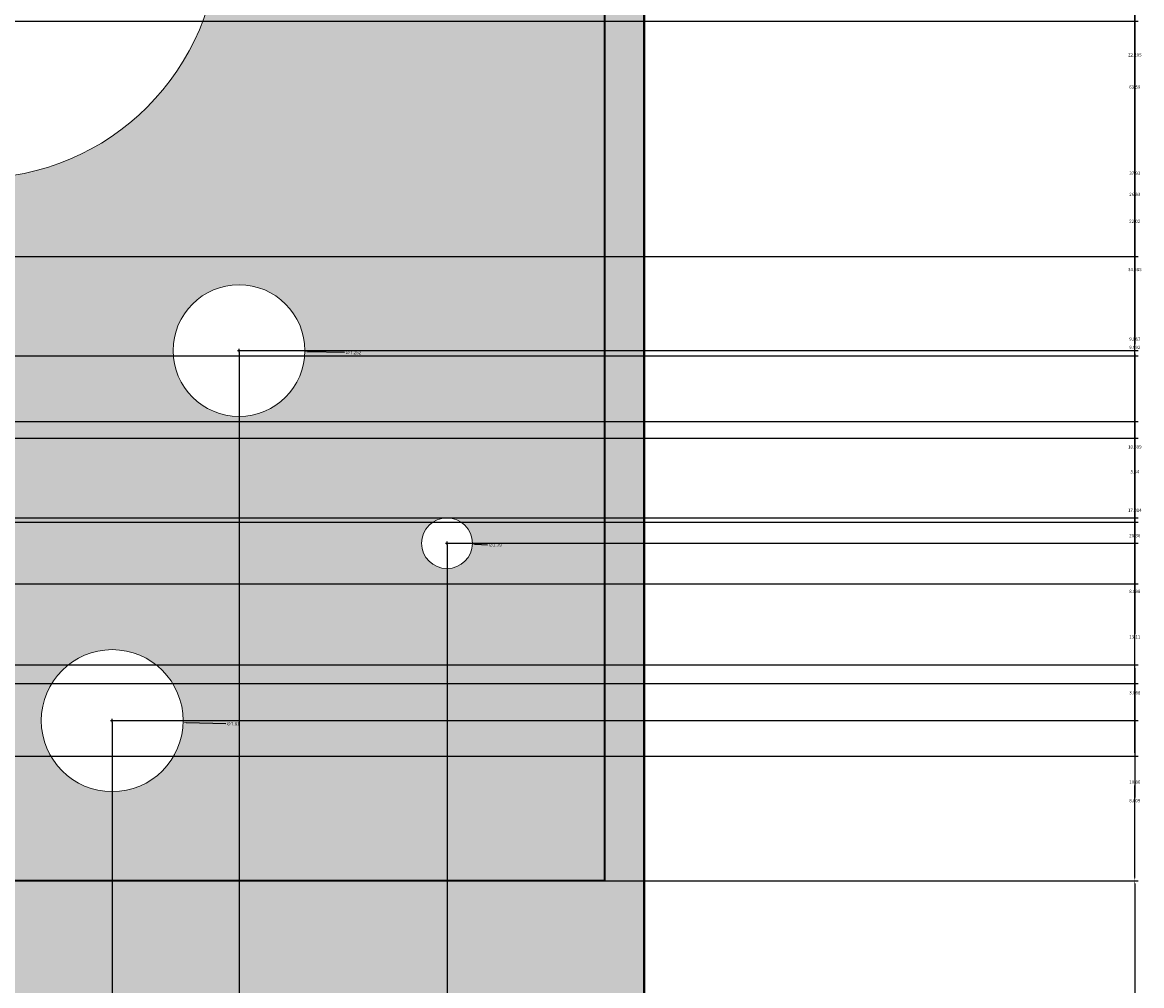
# Model space of a CAD drawing. Units: inches. Extents: x 73 to 607, y 92 to 651.
# Tile 10 of 18: x 546 to 607, y 169 to 222. Entities that reach past the tile are written whole.
import ezdxf

# ---------------------------------------------------------------- set-up
doc = ezdxf.new("R2010")
doc.units = ezdxf.units.IN
doc.header["$MEASUREMENT"] = 0
for name, color, linetype, lineweight in [('A-ANNO-DIMS', 2, 'Continuous', 18), ('A-ELEV', 7, 'Continuous', 35), ('A-ELEV-PANL', 7, 'Continuous', 18), ('A-ELEV-PATT-BKGD', 252, 'Continuous', 13), ('A-ELEV-PATT-SHAD', 8, 'Continuous', 13), ('A-ELEV-PATT-WOOD', 32, 'Continuous', 13)]:
    doc.layers.add(name, color=color, linetype=linetype, lineweight=lineweight)
doc.styles.get("Standard").update_dxf_attribs({"font": 'arial.ttf'})
doc.dimstyles.get("Standard").update_dxf_attribs({"dimtxt": 0.18, "dimasz": 0.18, "dimexe": 0.18, "dimexo": 0.0625, "dimgap": 0.09, "dimtad": 0, "dimtih": 1, "dimtoh": 1, "dimdec": 4, "dimzin": 0, "dimdsep": 46, "dimtxsty": 'Standard', "dimcen": 0.09, "dimadec": 0, "dimazin": 0, "dimtfac": 1, "dimtdec": 4, "dimtofl": 0, "dimtmove": 0, "dimatfit": 3, "dimfxl": 1, "dimtolj": 1, "dimtzin": 0, "dimarcsym": 0})

# ---------------------------------------------------------------- blocks, each defined once
blk = doc.blocks.new('*D15')
at = {"layer": 'A-ANNO-DIMS', "color": 0, "lineweight": -2, "transparency": 16777216}
for p, q in [((454.767, 174.802), (607.278, 174.802)), ((607.098, 174.622), (607.098, 159.185)), ((607.098, 143.384), (607.098, 158.821)), ((580.161, 143.204), (607.278, 143.204))]:
    blk.add_line(p, q, dxfattribs=at)
at = {"layer": 'A-ANNO-DIMS', "color": 0, "transparency": 16777216}
for points in [[(607.068, 174.622), (607.128, 174.622), (607.098, 174.802)], [(607.068, 143.384), (607.128, 143.384), (607.098, 143.204)]]:
    blk.add_solid(points, dxfattribs=at)
at = {"layer": 'Defpoints', "color": 0, "transparency": 16777216}
for p in [(454.705, 174.802), (607.098, 174.802), (580.098, 143.204)]:
    blk.add_point(p, dxfattribs=at)
at = {"layer": 'A-ANNO-DIMS', "color": 0, "transparency": 16777216, "insert": (607.098, 159.003), "char_height": 0.18, "attachment_point": 5}
blk.add_mtext('\\A1;31.6', dxfattribs=at)
blk = doc.blocks.new('*D16')
at = {"layer": 'A-ANNO-DIMS', "color": 0, "lineweight": -2, "transparency": 16777216}
for p, q in [((431.133, 185.662), (607.278, 185.662)), ((607.098, 185.482), (607.098, 180.414)), ((607.098, 174.982), (607.098, 180.05)), ((454.767, 174.802), (607.278, 174.802))]:
    blk.add_line(p, q, dxfattribs=at)
at = {"layer": 'A-ANNO-DIMS', "color": 0, "transparency": 16777216}
for points in [[(607.068, 185.482), (607.128, 185.482), (607.098, 185.662)], [(607.068, 174.982), (607.128, 174.982), (607.098, 174.802)]]:
    blk.add_solid(points, dxfattribs=at)
at = {"layer": 'Defpoints', "color": 0, "transparency": 16777216}
for p in [(431.07, 185.662), (607.098, 185.662), (454.705, 174.802)]:
    blk.add_point(p, dxfattribs=at)
at = {"layer": 'A-ANNO-DIMS', "color": 0, "transparency": 16777216, "insert": (607.098, 180.232), "char_height": 0.18, "attachment_point": 5}
blk.add_mtext('\\A1;10.86', dxfattribs=at)
blk = doc.blocks.new('*D17')
at = {"layer": 'A-ANNO-DIMS', "color": 0, "lineweight": -2, "transparency": 16777216}
for p, q in [((580.161, 262.302), (607.278, 262.302)), ((607.098, 262.122), (607.098, 224.164)), ((607.098, 185.842), (607.098, 223.8)), ((431.133, 185.662), (607.278, 185.662))]:
    blk.add_line(p, q, dxfattribs=at)
at = {"layer": 'A-ANNO-DIMS', "color": 0, "transparency": 16777216}
for points in [[(607.068, 262.122), (607.128, 262.122), (607.098, 262.302)], [(607.068, 185.842), (607.128, 185.842), (607.098, 185.662)]]:
    blk.add_solid(points, dxfattribs=at)
at = {"layer": 'Defpoints', "color": 0, "transparency": 16777216}
for p in [(580.098, 262.302), (607.098, 262.302), (431.07, 185.662)]:
    blk.add_point(p, dxfattribs=at)
at = {"layer": 'A-ANNO-DIMS', "color": 0, "transparency": 16777216, "insert": (607.098, 223.982), "char_height": 0.18, "attachment_point": 5}
blk.add_mtext('\\A1;76.64', dxfattribs=at)
blk = doc.blocks.new('*D94')
at = {"layer": 'A-ANNO-DIMS', "color": 0, "lineweight": -2, "transparency": 16777216}
for p, q in [((377.023, 209.143), (607.278, 209.143)), ((607.098, 208.963), (607.098, 204.329)), ((607.098, 199.331), (607.098, 203.965)), ((363.319, 199.151), (607.278, 199.151))]:
    blk.add_line(p, q, dxfattribs=at)
at = {"layer": 'A-ANNO-DIMS', "color": 0, "transparency": 16777216}
for points in [[(607.068, 208.963), (607.128, 208.963), (607.098, 209.143)], [(607.068, 199.331), (607.128, 199.331), (607.098, 199.151)]]:
    blk.add_solid(points, dxfattribs=at)
at = {"layer": 'Defpoints', "color": 0, "transparency": 16777216}
for p in [(376.96, 209.143), (363.256, 199.151), (607.098, 199.151)]:
    blk.add_point(p, dxfattribs=at)
at = {"layer": 'A-ANNO-DIMS', "color": 0, "transparency": 16777216, "insert": (607.098, 204.147), "char_height": 0.18, "attachment_point": 5}
blk.add_mtext('\\A1;9.992', dxfattribs=at)
blk = doc.blocks.new('*D95')
at = {"layer": 'A-ANNO-DIMS', "color": 0, "lineweight": -2, "transparency": 16777216}
for p, q in [((363.874, 225.982), (607.278, 225.982)), ((607.098, 225.802), (607.098, 212.749)), ((607.098, 199.331), (607.098, 212.385)), ((363.319, 199.151), (607.278, 199.151))]:
    blk.add_line(p, q, dxfattribs=at)
at = {"layer": 'A-ANNO-DIMS', "color": 0, "transparency": 16777216}
for points in [[(607.068, 225.802), (607.128, 225.802), (607.098, 225.982)], [(607.068, 199.331), (607.128, 199.331), (607.098, 199.151)]]:
    blk.add_solid(points, dxfattribs=at)
at = {"layer": 'Defpoints', "color": 0, "transparency": 16777216}
for p in [(363.812, 225.982), (607.098, 225.982), (363.256, 199.151)]:
    blk.add_point(p, dxfattribs=at)
at = {"layer": 'A-ANNO-DIMS', "color": 0, "transparency": 16777216, "insert": (607.098, 212.567), "char_height": 0.18, "attachment_point": 5}
blk.add_mtext('\\A1;26.83', dxfattribs=at)
blk = doc.blocks.new('*D97')
at = {"layer": 'A-ANNO-DIMS', "color": 0, "lineweight": -2, "transparency": 16777216}
for p, q in [((387.579, 200.076), (607.278, 200.076)), ((607.098, 199.896), (607.098, 197.488)), ((607.098, 194.717), (607.098, 197.125)), ((396.755, 194.537), (607.278, 194.537))]:
    blk.add_line(p, q, dxfattribs=at)
at = {"layer": 'A-ANNO-DIMS', "color": 0, "transparency": 16777216}
for points in [[(607.068, 199.896), (607.128, 199.896), (607.098, 200.076)], [(607.068, 194.717), (607.128, 194.717), (607.098, 194.537)]]:
    blk.add_solid(points, dxfattribs=at)
at = {"layer": 'Defpoints', "color": 0, "transparency": 16777216}
for p in [(387.516, 200.076), (607.098, 200.076), (396.692, 194.537)]:
    blk.add_point(p, dxfattribs=at)
at = {"layer": 'A-ANNO-DIMS', "color": 0, "transparency": 16777216, "insert": (607.098, 197.306), "char_height": 0.18, "attachment_point": 5}
blk.add_mtext('\\A1;5.54', dxfattribs=at)
blk = doc.blocks.new('*D98')
at = {"layer": 'A-ANNO-DIMS', "color": 0, "lineweight": -2, "transparency": 16777216}
for p, q in [((377.023, 209.143), (607.278, 209.143)), ((607.098, 208.963), (607.098, 204.792)), ((607.098, 200.256), (607.098, 204.428)), ((387.579, 200.076), (607.278, 200.076))]:
    blk.add_line(p, q, dxfattribs=at)
at = {"layer": 'A-ANNO-DIMS', "color": 0, "transparency": 16777216}
for points in [[(607.068, 208.963), (607.128, 208.963), (607.098, 209.143)], [(607.068, 200.256), (607.128, 200.256), (607.098, 200.076)]]:
    blk.add_solid(points, dxfattribs=at)
at = {"layer": 'Defpoints', "color": 0, "transparency": 16777216}
for p in [(376.96, 209.143), (607.098, 209.143), (387.516, 200.076)]:
    blk.add_point(p, dxfattribs=at)
at = {"layer": 'A-ANNO-DIMS', "color": 0, "transparency": 16777216, "insert": (607.098, 204.61), "char_height": 0.18, "attachment_point": 5}
blk.add_mtext('\\A1;9.067', dxfattribs=at)
blk = doc.blocks.new('*D99')
at = {"layer": 'A-ANNO-DIMS', "color": 0, "lineweight": -2, "transparency": 16777216}
for p, q in [((373.319, 231.348), (607.278, 231.348)), ((607.098, 231.168), (607.098, 220.428)), ((607.098, 209.323), (607.098, 220.064)), ((377.023, 209.143), (607.278, 209.143))]:
    blk.add_line(p, q, dxfattribs=at)
at = {"layer": 'A-ANNO-DIMS', "color": 0, "transparency": 16777216}
for points in [[(607.068, 231.168), (607.128, 231.168), (607.098, 231.348)], [(607.068, 209.323), (607.128, 209.323), (607.098, 209.143)]]:
    blk.add_solid(points, dxfattribs=at)
at = {"layer": 'Defpoints', "color": 0, "transparency": 16777216}
for p in [(373.257, 231.348), (607.098, 231.348), (376.96, 209.143)]:
    blk.add_point(p, dxfattribs=at)
at = {"layer": 'A-ANNO-DIMS', "color": 0, "transparency": 16777216, "insert": (607.098, 220.246), "char_height": 0.18, "attachment_point": 5}
blk.add_mtext('\\A1;22.205', dxfattribs=at)
blk = doc.blocks.new('*D100')
at = {"layer": 'A-ANNO-DIMS', "color": 0, "lineweight": -2, "transparency": 16777216}
for p, q in [((382.949, 222.096), (607.278, 222.096)), ((607.098, 221.916), (607.098, 211.268)), ((607.098, 200.256), (607.098, 210.904)), ((387.579, 200.076), (607.278, 200.076))]:
    blk.add_line(p, q, dxfattribs=at)
at = {"layer": 'A-ANNO-DIMS', "color": 0, "transparency": 16777216}
for points in [[(607.068, 221.916), (607.128, 221.916), (607.098, 222.096)], [(607.068, 200.256), (607.128, 200.256), (607.098, 200.076)]]:
    blk.add_solid(points, dxfattribs=at)
at = {"layer": 'Defpoints', "color": 0, "transparency": 16777216}
for p in [(382.886, 222.096), (607.098, 222.096), (387.516, 200.076)]:
    blk.add_point(p, dxfattribs=at)
at = {"layer": 'A-ANNO-DIMS', "color": 0, "transparency": 16777216, "insert": (607.098, 211.086), "char_height": 0.18, "attachment_point": 5}
blk.add_mtext('\\A1;22.02', dxfattribs=at)
blk = doc.blocks.new('*D116')
at = {"layer": 'A-ANNO-DIMS', "color": 0, "lineweight": -2, "transparency": 16777216}
for p, q in [((531.568, 203.63), (531.568, 116.024)), ((550.829, 183.548), (550.829, 116.024)), ((531.748, 116.204), (540.814, 116.204)), ((550.649, 116.204), (541.584, 116.204))]:
    blk.add_line(p, q, dxfattribs=at)
at = {"layer": 'A-ANNO-DIMS', "color": 0, "transparency": 16777216}
for points in [[(531.748, 116.234), (531.748, 116.174), (531.568, 116.204)], [(550.649, 116.234), (550.649, 116.174), (550.829, 116.204)]]:
    blk.add_solid(points, dxfattribs=at)
at = {"layer": 'Defpoints', "color": 0, "transparency": 16777216}
for p in [(531.568, 203.693), (550.829, 183.611), (550.829, 116.204)]:
    blk.add_point(p, dxfattribs=at)
at = {"layer": 'A-ANNO-DIMS', "color": 0, "transparency": 16777216, "insert": (541.199, 116.204), "char_height": 0.18, "attachment_point": 5}
blk.add_mtext('\\A1;19.26', dxfattribs=at)
blk = doc.blocks.new('*D117')
at = {"layer": 'A-ANNO-DIMS', "color": 0, "lineweight": -2, "transparency": 16777216}
for p, q in [((557.807, 203.909), (557.807, 116.024)), ((550.829, 183.548), (550.829, 116.024)), ((551.009, 116.204), (553.924, 116.204)), ((557.627, 116.204), (554.712, 116.204))]:
    blk.add_line(p, q, dxfattribs=at)
at = {"layer": 'A-ANNO-DIMS', "color": 0, "transparency": 16777216}
for points in [[(551.009, 116.234), (551.009, 116.174), (550.829, 116.204)], [(557.627, 116.234), (557.627, 116.174), (557.807, 116.204)]]:
    blk.add_solid(points, dxfattribs=at)
at = {"layer": 'Defpoints', "color": 0, "transparency": 16777216}
for p in [(557.807, 203.972), (550.829, 183.611), (557.807, 116.204)]:
    blk.add_point(p, dxfattribs=at)
at = {"layer": 'A-ANNO-DIMS', "color": 0, "transparency": 16777216, "insert": (554.318, 116.204), "char_height": 0.18, "attachment_point": 5}
blk.add_mtext('\\A1;6.978', dxfattribs=at)
blk = doc.blocks.new('*D118')
at = {"layer": 'A-ANNO-DIMS', "color": 0, "lineweight": -2, "transparency": 16777216}
for p, q in [((557.807, 203.909), (557.807, 116.024)), ((569.252, 193.31), (569.252, 116.024)), ((557.987, 116.204), (563.074, 116.204)), ((569.072, 116.204), (563.985, 116.204))]:
    blk.add_line(p, q, dxfattribs=at)
at = {"layer": 'A-ANNO-DIMS', "color": 0, "transparency": 16777216}
for points in [[(557.987, 116.234), (557.987, 116.174), (557.807, 116.204)], [(569.072, 116.234), (569.072, 116.174), (569.252, 116.204)]]:
    blk.add_solid(points, dxfattribs=at)
at = {"layer": 'Defpoints', "color": 0, "transparency": 16777216}
for p in [(557.807, 203.972), (569.252, 193.373), (569.252, 116.204)]:
    blk.add_point(p, dxfattribs=at)
at = {"layer": 'A-ANNO-DIMS', "color": 0, "transparency": 16777216, "insert": (563.53, 116.204), "char_height": 0.18, "attachment_point": 5}
blk.add_mtext('\\A1;11.445', dxfattribs=at)
blk = doc.blocks.new('*D120')
at = {"layer": 'A-ANNO-DIMS', "color": 0, "lineweight": -2, "transparency": 16777216}
for p, q in [((468.546, 225.727), (607.278, 225.727)), ((607.098, 225.547), (607.098, 208.616)), ((607.098, 191.322), (607.098, 208.252)), ((469.942, 191.142), (607.278, 191.142))]:
    blk.add_line(p, q, dxfattribs=at)
at = {"layer": 'A-ANNO-DIMS', "color": 0, "transparency": 16777216}
for points in [[(607.068, 225.547), (607.128, 225.547), (607.098, 225.727)], [(607.068, 191.322), (607.128, 191.322), (607.098, 191.142)]]:
    blk.add_solid(points, dxfattribs=at)
at = {"layer": 'Defpoints', "color": 0, "transparency": 16777216}
for p in [(468.484, 225.727), (607.098, 225.727), (469.879, 191.142)]:
    blk.add_point(p, dxfattribs=at)
at = {"layer": 'A-ANNO-DIMS', "color": 0, "transparency": 16777216, "insert": (607.098, 208.434), "char_height": 0.18, "attachment_point": 5}
blk.add_mtext('\\A1;34.585', dxfattribs=at)
blk = doc.blocks.new('*D122')
at = {"layer": 'A-ANNO-DIMS', "color": 0, "lineweight": -2, "transparency": 16777216}
for p, q in [((509.021, 194.767), (607.278, 194.767)), ((607.098, 194.587), (607.098, 188.395)), ((607.098, 181.839), (607.098, 188.031)), ((492.831, 181.659), (607.278, 181.659))]:
    blk.add_line(p, q, dxfattribs=at)
at = {"layer": 'A-ANNO-DIMS', "color": 0, "transparency": 16777216}
for points in [[(607.068, 194.587), (607.128, 194.587), (607.098, 194.767)], [(607.068, 181.839), (607.128, 181.839), (607.098, 181.659)]]:
    blk.add_solid(points, dxfattribs=at)
at = {"layer": 'Defpoints', "color": 0, "transparency": 16777216}
for p in [(508.958, 194.767), (492.769, 181.659), (607.098, 181.659)]:
    blk.add_point(p, dxfattribs=at)
at = {"layer": 'A-ANNO-DIMS', "color": 0, "transparency": 16777216, "insert": (607.098, 188.213), "char_height": 0.18, "attachment_point": 5}
blk.add_mtext('\\A1;13.11', dxfattribs=at)
blk = doc.blocks.new('*D123')
at = {"layer": 'A-ANNO-DIMS', "color": 0, "lineweight": -2, "transparency": 16777216}
for p, q in [((550.891, 183.611), (607.278, 183.611)), ((607.098, 183.431), (607.098, 179.388)), ((607.098, 174.982), (607.098, 179.025)), ((577.987, 174.802), (607.278, 174.802))]:
    blk.add_line(p, q, dxfattribs=at)
at = {"layer": 'A-ANNO-DIMS', "color": 0, "transparency": 16777216}
for points in [[(607.068, 183.431), (607.128, 183.431), (607.098, 183.611)], [(607.068, 174.982), (607.128, 174.982), (607.098, 174.802)]]:
    blk.add_solid(points, dxfattribs=at)
at = {"layer": 'Defpoints', "color": 0, "transparency": 16777216}
for p in [(550.829, 183.611), (607.098, 183.611), (577.925, 174.802)]:
    blk.add_point(p, dxfattribs=at)
at = {"layer": 'A-ANNO-DIMS', "color": 0, "transparency": 16777216, "insert": (607.098, 179.207), "char_height": 0.18, "attachment_point": 5}
blk.add_mtext('\\A1;8.809', dxfattribs=at)
blk = doc.blocks.new('*D124')
at = {"layer": 'A-ANNO-DIMS', "color": 0, "lineweight": -2, "transparency": 16777216}
for p, q in [((523.815, 186.679), (607.278, 186.679)), ((607.098, 186.499), (607.098, 185.327)), ((607.098, 183.791), (607.098, 184.963)), ((550.891, 183.611), (607.278, 183.611))]:
    blk.add_line(p, q, dxfattribs=at)
at = {"layer": 'A-ANNO-DIMS', "color": 0, "transparency": 16777216}
for points in [[(607.068, 186.499), (607.128, 186.499), (607.098, 186.679)], [(607.068, 183.791), (607.128, 183.791), (607.098, 183.611)]]:
    blk.add_solid(points, dxfattribs=at)
at = {"layer": 'Defpoints', "color": 0, "transparency": 16777216}
for p in [(523.753, 186.679), (607.098, 186.679), (550.829, 183.611)]:
    blk.add_point(p, dxfattribs=at)
at = {"layer": 'A-ANNO-DIMS', "color": 0, "transparency": 16777216, "insert": (607.098, 185.145), "char_height": 0.18, "attachment_point": 5}
blk.add_mtext('\\A1;3.068', dxfattribs=at)
blk = doc.blocks.new('*D125')
at = {"layer": 'A-ANNO-DIMS', "color": 0, "lineweight": -2, "transparency": 16777216}
for p, q in [((509.021, 194.767), (607.278, 194.767)), ((607.098, 194.587), (607.098, 190.905)), ((607.098, 186.859), (607.098, 190.541)), ((523.815, 186.679), (607.278, 186.679))]:
    blk.add_line(p, q, dxfattribs=at)
at = {"layer": 'A-ANNO-DIMS', "color": 0, "transparency": 16777216}
for points in [[(607.068, 194.587), (607.128, 194.587), (607.098, 194.767)], [(607.068, 186.859), (607.128, 186.859), (607.098, 186.679)]]:
    blk.add_solid(points, dxfattribs=at)
at = {"layer": 'Defpoints', "color": 0, "transparency": 16777216}
for p in [(508.958, 194.767), (607.098, 194.767), (523.753, 186.679)]:
    blk.add_point(p, dxfattribs=at)
at = {"layer": 'A-ANNO-DIMS', "color": 0, "transparency": 16777216, "insert": (607.098, 190.723), "char_height": 0.18, "attachment_point": 5}
blk.add_mtext('\\A1;8.088', dxfattribs=at)
blk = doc.blocks.new('*D126')
at = {"layer": 'A-ANNO-DIMS', "color": 0, "lineweight": -2, "transparency": 16777216}
for p, q in [((509.3, 232.7), (607.278, 232.7)), ((607.098, 232.52), (607.098, 213.915)), ((607.098, 194.947), (607.098, 213.552)), ((509.021, 194.767), (607.278, 194.767))]:
    blk.add_line(p, q, dxfattribs=at)
at = {"layer": 'A-ANNO-DIMS', "color": 0, "transparency": 16777216}
for points in [[(607.068, 232.52), (607.128, 232.52), (607.098, 232.7)], [(607.068, 194.947), (607.128, 194.947), (607.098, 194.767)]]:
    blk.add_solid(points, dxfattribs=at)
at = {"layer": 'Defpoints', "color": 0, "transparency": 16777216}
for p in [(509.238, 232.7), (607.098, 232.7), (508.958, 194.767)]:
    blk.add_point(p, dxfattribs=at)
at = {"layer": 'A-ANNO-DIMS', "color": 0, "transparency": 16777216, "insert": (607.098, 213.733), "char_height": 0.18, "attachment_point": 5}
blk.add_mtext('\\A1;37.93', dxfattribs=at)
blk = doc.blocks.new('*D127')
at = {"layer": 'A-ANNO-DIMS', "color": 0, "lineweight": -2, "transparency": 16777216}
for p, q in [((524.094, 250.271), (607.278, 250.271)), ((607.098, 250.091), (607.098, 218.657)), ((607.098, 186.859), (607.098, 218.293)), ((523.815, 186.679), (607.278, 186.679))]:
    blk.add_line(p, q, dxfattribs=at)
at = {"layer": 'A-ANNO-DIMS', "color": 0, "transparency": 16777216}
for points in [[(607.068, 250.091), (607.128, 250.091), (607.098, 250.271)], [(607.068, 186.859), (607.128, 186.859), (607.098, 186.679)]]:
    blk.add_solid(points, dxfattribs=at)
at = {"layer": 'Defpoints', "color": 0, "transparency": 16777216}
for p in [(524.032, 250.271), (607.098, 250.271), (523.753, 186.679)]:
    blk.add_point(p, dxfattribs=at)
at = {"layer": 'A-ANNO-DIMS', "color": 0, "transparency": 16777216, "insert": (607.098, 218.475), "char_height": 0.18, "attachment_point": 5}
blk.add_mtext('\\A1;63.59', dxfattribs=at)
blk = doc.blocks.new('*D128')
at = {"layer": 'A-ANNO-DIMS', "color": 0, "lineweight": -2, "transparency": 16777216}
for p, q in [((531.631, 203.693), (607.278, 203.693)), ((607.098, 203.513), (607.098, 195.368)), ((607.098, 186.859), (607.098, 195.004)), ((523.815, 186.679), (607.278, 186.679))]:
    blk.add_line(p, q, dxfattribs=at)
at = {"layer": 'A-ANNO-DIMS', "color": 0, "transparency": 16777216}
for points in [[(607.068, 203.513), (607.128, 203.513), (607.098, 203.693)], [(607.068, 186.859), (607.128, 186.859), (607.098, 186.679)]]:
    blk.add_solid(points, dxfattribs=at)
at = {"layer": 'Defpoints', "color": 0, "transparency": 16777216}
for p in [(531.568, 203.693), (607.098, 203.693), (523.753, 186.679)]:
    blk.add_point(p, dxfattribs=at)
at = {"layer": 'A-ANNO-DIMS', "color": 0, "transparency": 16777216, "insert": (607.098, 195.186), "char_height": 0.18, "attachment_point": 5}
blk.add_mtext('\\A1;17.014', dxfattribs=at)
blk = doc.blocks.new('*D129')
at = {"layer": 'A-ANNO-DIMS', "color": 0, "lineweight": -2, "transparency": 16777216}
for p, q in [((557.87, 203.972), (607.278, 203.972)), ((607.098, 203.792), (607.098, 193.973)), ((607.098, 183.791), (607.098, 193.609)), ((550.891, 183.611), (607.278, 183.611))]:
    blk.add_line(p, q, dxfattribs=at)
at = {"layer": 'A-ANNO-DIMS', "color": 0, "transparency": 16777216}
for points in [[(607.068, 203.792), (607.128, 203.792), (607.098, 203.972)], [(607.068, 183.791), (607.128, 183.791), (607.098, 183.611)]]:
    blk.add_solid(points, dxfattribs=at)
at = {"layer": 'Defpoints', "color": 0, "transparency": 16777216}
for p in [(557.807, 203.972), (607.098, 203.972), (550.829, 183.611)]:
    blk.add_point(p, dxfattribs=at)
at = {"layer": 'A-ANNO-DIMS', "color": 0, "transparency": 16777216, "insert": (607.098, 193.791), "char_height": 0.18, "attachment_point": 5}
blk.add_mtext('\\A1;20.36', dxfattribs=at)
blk = doc.blocks.new('*D130')
at = {"layer": 'A-ANNO-DIMS', "color": 0, "lineweight": -2, "transparency": 16777216}
for p, q in [((557.87, 203.972), (607.278, 203.972)), ((607.098, 203.792), (607.098, 198.854)), ((607.098, 193.553), (607.098, 198.49)), ((569.314, 193.373), (607.278, 193.373))]:
    blk.add_line(p, q, dxfattribs=at)
at = {"layer": 'A-ANNO-DIMS', "color": 0, "transparency": 16777216}
for points in [[(607.068, 203.792), (607.128, 203.792), (607.098, 203.972)], [(607.068, 193.553), (607.128, 193.553), (607.098, 193.373)]]:
    blk.add_solid(points, dxfattribs=at)
at = {"layer": 'Defpoints', "color": 0, "transparency": 16777216}
for p in [(557.807, 203.972), (569.252, 193.373), (607.098, 193.373)]:
    blk.add_point(p, dxfattribs=at)
at = {"layer": 'A-ANNO-DIMS', "color": 0, "transparency": 16777216, "insert": (607.098, 198.672), "char_height": 0.18, "attachment_point": 5}
blk.add_mtext('\\A1;10.599', dxfattribs=at)
blk = doc.blocks.new('*D163')
at = {"layer": 'A-ANNO-DIMS', "color": 0, "lineweight": -2, "transparency": 16777216}
for p, q in [((557.717, 203.972), (557.897, 203.972)), ((557.807, 203.882), (557.807, 204.062)), ((563.608, 203.863), (561.612, 203.9))]:
    blk.add_line(p, q, dxfattribs=at)
at = {"layer": 'A-ANNO-DIMS', "color": 0, "transparency": 16777216}
blk.add_solid([(561.613, 203.93), (561.612, 203.87), (561.432, 203.904)], dxfattribs=at)
at = {"layer": 'Defpoints', "color": 0, "transparency": 16777216}
for p in [(554.182, 204.039), (561.432, 203.904)]:
    blk.add_point(p, dxfattribs=at)
at = {"layer": 'A-ANNO-DIMS', "color": 0, "transparency": 16777216, "insert": (564.098, 203.863), "char_height": 0.18, "attachment_point": 5}
blk.add_mtext('\\A1;∅7.252', dxfattribs=at)
blk = doc.blocks.new('*D166')
at = {"layer": 'A-ANNO-DIMS', "color": 0, "lineweight": -2, "transparency": 16777216}
for p, q in [((569.252, 193.283), (569.252, 193.463)), ((569.162, 193.373), (569.342, 193.373)), ((571.482, 193.268), (570.826, 193.299))]:
    blk.add_line(p, q, dxfattribs=at)
at = {"layer": 'A-ANNO-DIMS', "color": 0, "transparency": 16777216}
blk.add_solid([(570.827, 193.329), (570.824, 193.269), (570.646, 193.307)], dxfattribs=at)
at = {"layer": 'Defpoints', "color": 0, "transparency": 16777216}
for p in [(567.858, 193.439), (570.646, 193.307)]:
    blk.add_point(p, dxfattribs=at)
at = {"layer": 'A-ANNO-DIMS', "color": 0, "transparency": 16777216, "insert": (571.904, 193.268), "char_height": 0.18, "attachment_point": 5}
blk.add_mtext('\\A1;∅2.79', dxfattribs=at)
blk = doc.blocks.new('*D169')
at = {"layer": 'A-ANNO-DIMS', "color": 0, "lineweight": -2, "transparency": 16777216}
for p, q in [((550.739, 183.611), (550.919, 183.611)), ((550.829, 183.521), (550.829, 183.701)), ((557.074, 183.436), (554.912, 183.497))]:
    blk.add_line(p, q, dxfattribs=at)
at = {"layer": 'A-ANNO-DIMS', "color": 0, "transparency": 16777216}
blk.add_solid([(554.913, 183.527), (554.911, 183.467), (554.732, 183.502)], dxfattribs=at)
at = {"layer": 'Defpoints', "color": 0, "transparency": 16777216}
for p in [(546.926, 183.72), (554.732, 183.502)]:
    blk.add_point(p, dxfattribs=at)
at = {"layer": 'A-ANNO-DIMS', "color": 0, "transparency": 16777216, "insert": (557.478, 183.436), "char_height": 0.18, "attachment_point": 5}
blk.add_mtext('\\A1;∅7.81', dxfattribs=at)

msp = doc.modelspace()

# ---------------------------------------------------------------- hatches: boundary and pattern name
at = {"layer": 'A-ELEV-PATT-BKGD'}
h = msp.add_hatch(color=256, dxfattribs=at)
h.dxf.hatch_style = 1
h.paths.add_polyline_path([(321.3008, 479.2042), (312.3008, 479.2042), (312.3008, 478.7576), (312.3008, 412.636), (321.3008, 412.636)])
h.paths.add_polyline_path([(312.3008, 504.7576), (256.4726, 504.7576), (256.4726, 503.4576), (312.3008, 503.4576)], flags=17)
h.paths.add_polyline_path([(321.3008, 543.1576), (321.3008, 552.1576), (320.3257, 552.1576), (312.3008, 552.1576), (256.4726, 552.1576), (256.4726, 543.1576), (312.3008, 543.1576), (312.3008, 479.2042), (321.3008, 479.2042)])
h.paths.add_polyline_path([(451.5214, 412.636), (256.4726, 412.636), (256.4726, 403.636), (442.5214, 403.636), (442.5214, 320.2042), (206.1343, 320.2042), (206.1343, 320.9135), (206.1343, 403.636), (256.4726, 403.636), (256.4726, 412.636), (201.6343, 412.636), (201.6343, 320.9135), (201.6343, 320.2042), (201.6343, 311.2042), (256.4726, 311.2042), (451.5214, 311.2042)])
h.paths.add_polyline_path([(431.07, 258.6914), (369.5339, 258.6914), (369.5339, 247.4054), (396.692, 247.4054), (425.07, 247.4054), (425.07, 194.7312), (396.692, 194.6197), (396.692, 194.5366), (369.5339, 194.5366), (369.5339, 185.6619), (431.07, 185.6619)])
h.paths.add_polyline_path([(580.0983, 262.3024), (451.5214, 262.3024), (451.5214, 143.2042), (580.0983, 143.2042)])
h.paths.add_polyline_path([(454.7049, 174.802), (454.7049, 256.6321), (577.9249, 256.6321), (577.9249, 174.802)], flags=16)
h.paths.add_polyline_path([(465.9716, 191.1416, -1), (473.7874, 191.1416, -1)], flags=0)
h.paths.add_polyline_path([(490.5373, 181.6586, -1), (494.9999, 181.6586, -1)], flags=0)
h.paths.add_polyline_path([(476.2996, 209.8287, -1), (500.5844, 209.8287, -1)], flags=0)
h.paths.add_polyline_path([(505.3326, 194.7675, -1), (512.5843, 194.7675, -1)], flags=0)
h.paths.add_polyline_path([(520.9613, 186.679, -1), (526.544, 186.679, -1)], flags=0)
h.paths.add_polyline_path([(466.8103, 225.7267, -1), (470.1573, 225.7267, -1)], flags=0)
h.paths.add_polyline_path([(527.1059, 203.6926, -1), (536.0311, 203.6926, -1)], flags=0)
h.paths.add_polyline_path([(504.775, 232.6995, -1), (513.7002, 232.6995, -1)], flags=0)
h.paths.add_polyline_path([(546.9241, 183.611, -1), (554.7336, 183.611, -1)], flags=0)
h.paths.add_polyline_path([(459.5544, 243.856, -1), (466.8061, 243.856, -1)], flags=0)
h.paths.add_polyline_path([(476.3045, 246.924, -1), (488.5767, 246.924, -1)], flags=0)
h.paths.add_polyline_path([(529.9044, 226.8424, -1), (556.68, 226.8424, -1)], flags=0)
h.paths.add_polyline_path([(554.1814, 203.9716, -1), (561.4331, 203.9716, -1)], flags=0)
h.paths.add_polyline_path([(567.8561, 193.3729, -1), (570.6475, 193.3729, -1)], flags=0)
h.paths.add_polyline_path([(522.3584, 250.271, -1), (525.7053, 250.271, -1)], flags=0)
h.paths.add_polyline_path([(561.9965, 245.2506, -1), (567.5748, 245.2506, -1)], flags=0)
h.paths.add_polyline_path([(347.8686, 194.5366), (341.8686, 194.5366), (341.8686, 194.5452), (314.0144, 194.5452), (314.0144, 188.5452), (347.8686, 188.5452)])
h.paths.add_polyline_path([(347.8686, 253.4054), (314.0144, 253.4054), (314.0144, 247.4054), (341.8686, 247.4054), (347.8686, 247.4054)])
h.paths.add_polyline_path([(304.3559, 253.4054), (298.3559, 253.4054), (298.3559, 188.5452), (304.3559, 188.5452)])
h.paths.add_polyline_path([(450.6603, 552.1576), (369.9727, 552.1576), (369.9727, 479.2042), (374.4727, 479.2042), (374.4727, 547.6576), (446.1603, 547.6576), (446.1603, 479.2042), (450.6603, 479.2042)])
h.paths.add_polyline_path([(374.4727, 479.2042), (369.9727, 479.2042), (369.9727, 465.0632), (374.4727, 465.0632)])
h.paths.add_polyline_path([(450.6603, 479.2042), (446.1603, 479.2042), (446.1603, 465.0632), (450.6603, 465.0632)])
h.paths.add_polyline_path([(256.4726, 281.6039), (109.0983, 281.6039), (100.0983, 281.6039), (100.0983, 167.2042), (100.0983, 143.2042), (109.0983, 143.2042), (109.0983, 167.2042), (109.0983, 272.6039), (256.4726, 272.6039)])
at = {"layer": 'A-ELEV-PATT-SHAD'}
h = msp.add_hatch(color=256, dxfattribs=at)
h.dxf.hatch_style = 1
h.paths.add_polyline_path([(451.5214, 412.636), (256.4726, 412.636), (256.4726, 403.636), (442.5214, 403.636), (442.5214, 320.2042), (206.1343, 320.2042), (206.1343, 320.9135), (206.1343, 403.636), (256.4726, 403.636), (256.4726, 412.636), (201.6343, 412.636), (201.6343, 320.9135), (201.6343, 320.2042), (201.6343, 311.2042), (256.4726, 311.2042), (451.5214, 311.2042)])
h.paths.add_polyline_path([(580.0983, 262.3024), (451.5214, 262.3024), (451.5214, 143.2042), (580.0983, 143.2042)])
h.paths.add_polyline_path([(454.7049, 174.802), (454.7049, 256.6321), (577.9249, 256.6321), (577.9249, 174.802)], flags=16)
h.paths.add_polyline_path([(465.9716, 191.1416, -1), (473.7874, 191.1416, -1)], flags=0)
h.paths.add_polyline_path([(490.5373, 181.6586, -1), (494.9999, 181.6586, -1)], flags=0)
h.paths.add_polyline_path([(476.2996, 209.8287, -1), (500.5844, 209.8287, -1)], flags=0)
h.paths.add_polyline_path([(505.3326, 194.7675, -1), (512.5843, 194.7675, -1)], flags=0)
h.paths.add_polyline_path([(520.9613, 186.679, -1), (526.544, 186.679, -1)], flags=0)
h.paths.add_polyline_path([(466.8103, 225.7267, -1), (470.1573, 225.7267, -1)], flags=0)
h.paths.add_polyline_path([(527.1059, 203.6926, -1), (536.0311, 203.6926, -1)], flags=0)
h.paths.add_polyline_path([(459.5544, 243.856, -1), (466.8061, 243.856, -1)], flags=0)
h.paths.add_polyline_path([(504.775, 232.6995, -1), (513.7002, 232.6995, -1)], flags=0)
h.paths.add_polyline_path([(476.3045, 246.924, -1), (488.5767, 246.924, -1)], flags=0)
h.paths.add_polyline_path([(546.9241, 183.611, -1), (554.7336, 183.611, -1)], flags=0)
h.paths.add_polyline_path([(529.9044, 226.8424, -1), (556.68, 226.8424, -1)], flags=0)
h.paths.add_polyline_path([(554.1814, 203.9716, -1), (561.4331, 203.9716, -1)], flags=0)
h.paths.add_polyline_path([(522.3584, 250.271, -1), (525.7053, 250.271, -1)], flags=0)
h.paths.add_polyline_path([(567.8561, 193.3729, -1), (570.6475, 193.3729, -1)], flags=0)
h.paths.add_polyline_path([(561.9965, 245.2506, -1), (567.5748, 245.2506, -1)], flags=0)
h.paths.add_polyline_path([(431.07, 258.6914), (369.5339, 258.6914), (369.5339, 247.4054), (396.692, 247.4054), (425.07, 247.4054), (425.07, 194.7312), (396.692, 194.6197), (396.692, 194.5366), (369.5339, 194.5366), (369.5339, 185.6619), (431.07, 185.6619)])
h.paths.add_polyline_path([(347.8686, 253.4054), (314.0144, 253.4054), (314.0144, 247.4054), (341.8686, 247.4054), (347.8686, 247.4054)])
h.paths.add_polyline_path([(304.3559, 253.4054), (298.3559, 253.4054), (298.3559, 188.5452), (304.3559, 188.5452)])
h.paths.add_polyline_path([(347.8686, 194.5366), (341.8686, 194.5366), (341.8686, 194.5452), (314.0144, 194.5452), (314.0144, 188.5452), (347.8686, 188.5452)])
at = {"layer": 'A-ELEV-PATT-WOOD'}
h = msp.add_hatch(color=256, dxfattribs=at)
h.dxf.hatch_style = 1
h.paths.add_polyline_path([(577.9249, 256.6321), (454.7049, 256.6321), (454.7049, 174.802), (577.9249, 174.802)])
h.paths.add_polyline_path([(476.2996, 209.8287, -1), (500.5844, 209.8287, -1)], flags=16)
h.paths.add_polyline_path([(473.7874, 191.1416, -1), (465.9716, 191.1416, -1)], flags=16)
h.paths.add_polyline_path([(466.8103, 225.7267, -1), (470.1573, 225.7267, -1)], flags=16)
h.paths.add_polyline_path([(459.5544, 243.856, -1), (466.8061, 243.856, -1)], flags=16)
h.paths.add_polyline_path([(494.9999, 181.6586, -1), (490.5373, 181.6586, -1)], flags=16)
h.paths.add_polyline_path([(476.3045, 246.924, -1), (488.5767, 246.924, -1)], flags=16)
h.paths.add_polyline_path([(512.5843, 194.7675, -1), (505.3326, 194.7675, -1)], flags=16)
h.paths.add_polyline_path([(504.775, 232.6995, -1), (513.7002, 232.6995, -1)], flags=16)
h.paths.add_polyline_path([(526.544, 186.679, -1), (520.9613, 186.679, -1)], flags=16)
h.paths.add_polyline_path([(536.0311, 203.6926, -1), (527.1059, 203.6926, -1)], flags=16)
h.paths.add_polyline_path([(529.9044, 226.8424, -1), (556.68, 226.8424, -1)], flags=16)
h.paths.add_polyline_path([(522.3584, 250.271, -1), (525.7053, 250.271, -1)], flags=16)
h.paths.add_polyline_path([(554.7336, 183.611, -1), (546.9241, 183.611, -1)], flags=16)
h.paths.add_polyline_path([(561.4331, 203.9716, -1), (554.1814, 203.9716, -1)], flags=16)
h.paths.add_polyline_path([(561.9965, 245.2506, -1), (567.5748, 245.2506, -1)], flags=16)
h.paths.add_polyline_path([(570.6475, 193.3729, -1), (567.8561, 193.3729, -1)], flags=16)

# ---------------------------------------------------------------- linework, layer by layer
at = {"layer": 'A-ELEV'}
msp.add_line((580.0983, 167.2042), (580.0983, 311.2042), dxfattribs=at)
for points in [[(580.0983, 143.2042), (451.5214, 143.2042), (451.5214, 262.3024), (580.0983, 262.3024)], [(454.7049, 256.6321), (577.9249, 256.6321), (577.9249, 174.802), (454.7049, 174.802)]]:
    msp.add_lwpolyline(points, close=True, dxfattribs=at)
at = {"layer": 'A-ELEV-PANL'}
for centre, radius in [((543.2922, 226.8424), 13.3878), ((557.8072, 203.9716), 3.6259), ((569.2518, 193.3729), 1.3957), ((550.8289, 183.611), 3.9048)]:
    msp.add_circle(centre, radius, dxfattribs=at)

# ---------------------------------------------------------------- dimensions: what is measured, and where the dimension line sits
at = {"layer": 'A-ANNO-DIMS'}
for base, p1, p2, override, picture, middle in [((607.0983, 262.3024), (431.07, 185.6619), (580.0983, 262.3024), {"dimdec": 2, "dimlfac": 1, "dimrnd": 0, "dimzin": 0, "dimdsep": 46, "dimlunit": 2}, '*D17', (607.0983, 223.9821)), ((607.0983, 250.271), (523.7527, 186.679), (524.0318, 250.271), {"dimdec": 2, "dimlfac": 1, "dimrnd": 0, "dimzin": 0, "dimdsep": 46, "dimlunit": 2}, '*D127', (607.0983, 218.475)), ((607.0983, 232.6995), (508.9585, 194.7675), (509.2376, 232.6995), {"dimdec": 2, "dimlfac": 1, "dimrnd": 0, "dimzin": 0, "dimdsep": 46, "dimlunit": 2}, '*D126', (607.0983, 213.7335)), ((607.0983, 231.3482), (376.9603, 209.1433), (373.2566, 231.3482), {"dimdec": 3, "dimlfac": 1, "dimrnd": 0, "dimzin": 0, "dimdsep": 46, "dimlunit": 2}, '*D99', (607.0983, 220.2458)), ((607.0983, 225.982), (363.2564, 199.1512), (363.8119, 225.982), {"dimdec": 2, "dimlfac": 1, "dimrnd": 0, "dimzin": 0, "dimdsep": 46, "dimlunit": 2}, '*D95', (607.0983, 212.5666)), ((607.0983, 225.7267), (469.8795, 191.1416), (468.4838, 225.7267), {"dimdec": 3, "dimlfac": 1, "dimrnd": 0, "dimzin": 0, "dimdsep": 46, "dimlunit": 2}, '*D120', (607.0983, 208.4342)), ((607.0983, 222.0962), (387.5161, 200.0764), (382.8864, 222.0962), {"dimdec": 2, "dimlfac": 1, "dimrnd": 0, "dimzin": 0, "dimdsep": 46, "dimlunit": 2}, '*D100', (607.0983, 211.0863)), ((607.0983, 199.1512), (376.9603, 209.1433), (363.2564, 199.1512), {"dimdec": 3, "dimlfac": 1, "dimrnd": 0, "dimzin": 0, "dimdsep": 46, "dimlunit": 2}, '*D94', (607.0983, 204.1472)), ((607.0983, 209.1433), (387.5161, 200.0764), (376.9603, 209.1433), {"dimdec": 3, "dimlfac": 1, "dimrnd": 0, "dimzin": 0, "dimdsep": 46, "dimlunit": 2}, '*D98', (607.0983, 204.6098)), ((607.0983, 203.9716), (550.8289, 183.611), (557.8072, 203.9716), {"dimdec": 2, "dimlfac": 1, "dimrnd": 0, "dimzin": 0, "dimdsep": 46, "dimlunit": 2}, '*D129', (607.0983, 193.7913)), ((607.0983, 193.3729), (557.8072, 203.9716), (569.2518, 193.3729), {"dimdec": 3, "dimlfac": 1, "dimrnd": 0, "dimzin": 0, "dimdsep": 46, "dimlunit": 2}, '*D130', (607.0983, 198.6722)), ((607.0983, 203.6926), (523.7527, 186.679), (531.5685, 203.6926), {"dimdec": 3, "dimlfac": 1, "dimrnd": 0, "dimzin": 0, "dimdsep": 46, "dimlunit": 2}, '*D128', (607.0983, 195.1858)), ((607.0983, 200.0764), (396.692, 194.5366), (387.5161, 200.0764), {"dimdec": 2, "dimlfac": 1, "dimrnd": 0, "dimzin": 0, "dimdsep": 46, "dimlunit": 2}, '*D97', (607.0983, 197.3065)), ((607.0983, 181.6586), (508.9585, 194.7675), (492.7686, 181.6586), {"dimdec": 2, "dimlfac": 1, "dimrnd": 0, "dimzin": 0, "dimdsep": 46, "dimlunit": 2}, '*D122', (607.0983, 188.213)), ((607.0983, 194.76746), (523.75269, 186.679), (508.95849, 194.76746), {"dimdec": 3, "dimlfac": 1, "dimrnd": 0, "dimzin": 0, "dimdsep": 46, "dimlunit": 2}, '*D125', (607.0983, 190.72323)), ((607.0983, 186.679), (550.8289, 183.611), (523.7527, 186.679), {"dimdec": 3, "dimlfac": 1, "dimrnd": 0, "dimzin": 0, "dimdsep": 46, "dimlunit": 2}, '*D124', (607.0983, 185.145)), ((607.0983, 185.6619), (454.7049, 174.802), (431.07, 185.6619), {"dimdec": 2, "dimlfac": 1, "dimrnd": 0, "dimzin": 0, "dimdsep": 46, "dimlunit": 2}, '*D16', (607.0983, 180.232)), ((607.0983, 183.611), (577.9249, 174.802), (550.8289, 183.611), {"dimdec": 3, "dimlfac": 1, "dimrnd": 0, "dimzin": 0, "dimdsep": 46, "dimlunit": 2}, '*D123', (607.0983, 179.2065)), ((607.0983, 174.802), (580.0983, 143.2042), (454.7049, 174.802), {"dimdec": 1, "dimlfac": 1, "dimrnd": 0, "dimzin": 0, "dimdsep": 46, "dimlunit": 2}, '*D15', (607.0983, 159.0031))]:
    dim = msp.add_linear_dim(base=base, p1=p1, p2=p2, angle=90, dimstyle='Standard', override=override, dxfattribs=at)
    dim.commit()
    dim.dimension.update_dxf_attribs({"geometry": picture, "text_midpoint": middle})
for base, p1, p2, override, picture, middle in [((557.8072, 116.2042), (550.8289, 183.611), (557.8072, 203.9716), {"dimdec": 3, "dimlfac": 1, "dimrnd": 0, "dimzin": 0, "dimdsep": 46, "dimlunit": 2}, '*D117', (554.3181, 116.2042)), ((569.2518, 116.2042), (557.8072, 203.9716), (569.2518, 193.3729), {"dimdec": 3, "dimlfac": 1, "dimrnd": 0, "dimzin": 0, "dimdsep": 46, "dimlunit": 2}, '*D118', (563.5295, 116.2042)), ((550.8289, 116.2042), (531.5685, 203.6926), (550.8289, 183.611), {"dimdec": 2, "dimlfac": 1, "dimrnd": 0, "dimzin": 0, "dimdsep": 46, "dimlunit": 2}, '*D116', (541.1987, 116.2042))]:
    dim = msp.add_linear_dim(base=base, p1=p1, p2=p2, dimstyle='Standard', override=override, dxfattribs=at)
    dim.commit()
    dim.dimension.update_dxf_attribs({"geometry": picture, "text_midpoint": middle})
for p1, p2, override, picture, middle in [((554.182, 204.0394), (561.4325, 203.9037), {"dimdec": 3, "dimlfac": 1, "dimrnd": 0, "dimzin": 0, "dimdsep": 46, "dimlunit": 2}, '*D163', (563.6076, 203.863)), ((567.8577, 193.4385), (570.646, 193.3073), {"dimdec": 2, "dimlfac": 1, "dimrnd": 0, "dimzin": 0, "dimdsep": 46, "dimlunit": 2}, '*D166', (571.4824, 193.2679)), ((546.9256, 183.72), (554.7321, 183.5019), {"dimdec": 2, "dimlfac": 1, "dimrnd": 0, "dimzin": 0, "dimdsep": 46, "dimlunit": 2}, '*D169', (557.0741, 183.4365))]:
    dim = msp.add_diameter_dim_2p(p1=p1, p2=p2, dimstyle='Standard', override=override, dxfattribs=at)
    dim.commit()
    dim.dimension.update_dxf_attribs({"geometry": picture, "text_midpoint": middle, "dimtype": 163})

doc.saveas('drawing.dxf')
